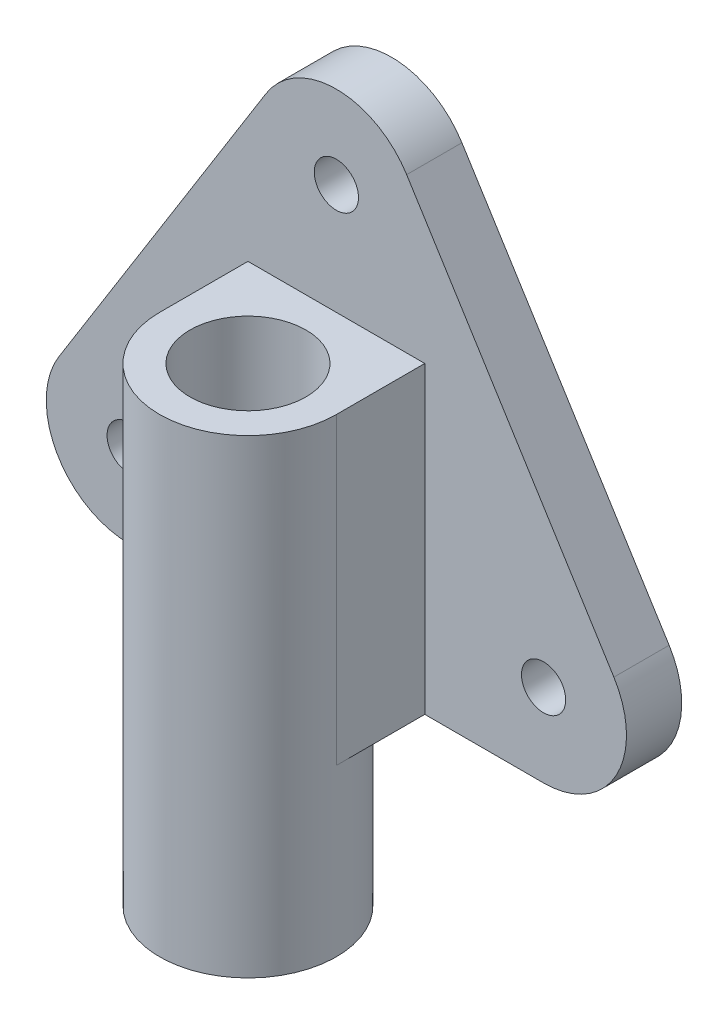
ISO-10303-21;
HEADER;
FILE_DESCRIPTION(('STEP AP214'),'2;1');
FILE_NAME('part.step','',(''),(''),'','','');
FILE_SCHEMA(('AUTOMOTIVE_DESIGN { 1 0 10303 214 1 1 1 1 }'));
ENDSEC;
DATA;
#1=APPLICATION_CONTEXT('core data for automotive mechanical design processes');
#2=APPLICATION_PROTOCOL_DEFINITION('international standard','automotive_design',2000,#1);
#3=PRODUCT_CONTEXT('',#1,'mechanical');
#4=PRODUCT('Part','Part','',(#3));
#5=PRODUCT_RELATED_PRODUCT_CATEGORY('part','',(#4));
#6=PRODUCT_DEFINITION_FORMATION('','',#4);
#7=PRODUCT_DEFINITION_CONTEXT('part definition',#1,'design');
#8=PRODUCT_DEFINITION('design','',#6,#7);
#9=PRODUCT_DEFINITION_SHAPE('','',#8);
#10=(LENGTH_UNIT() NAMED_UNIT(*) SI_UNIT(.MILLI.,.METRE.));
#11=(NAMED_UNIT(*) PLANE_ANGLE_UNIT() SI_UNIT($,.RADIAN.));
#12=(NAMED_UNIT(*) SI_UNIT($,.STERADIAN.) SOLID_ANGLE_UNIT());
#13=UNCERTAINTY_MEASURE_WITH_UNIT(LENGTH_MEASURE(1.E-05),#10,'distance_accuracy_value','');
#14=(GEOMETRIC_REPRESENTATION_CONTEXT(3) GLOBAL_UNCERTAINTY_ASSIGNED_CONTEXT((#13)) GLOBAL_UNIT_ASSIGNED_CONTEXT((#10,
#11,#12)) REPRESENTATION_CONTEXT('',''));
#15=CARTESIAN_POINT('',(0.,0.,0.));
#16=DIRECTION('',(0.,0.,1.));
#17=DIRECTION('',(1.,0.,0.));
#18=AXIS2_PLACEMENT_3D('',#15,#16,#17);
#19=CARTESIAN_POINT('',(0.,-75.,10.));
#20=DIRECTION('',(0.,1.,0.));
#21=DIRECTION('',(0.,0.,1.));
#22=AXIS2_PLACEMENT_3D('',#19,#20,#21);
#23=PLANE('',#22);
#24=CARTESIAN_POINT('',(0.,-75.,26.));
#25=DIRECTION('',(0.,-1.,0.));
#26=DIRECTION('',(0.,0.,-1.));
#27=AXIS2_PLACEMENT_3D('',#24,#25,#26);
#28=CIRCLE('',#27,16.);
#29=CARTESIAN_POINT('',(-16.,-75.,26.));
#30=VERTEX_POINT('',#29);
#31=CARTESIAN_POINT('',(16.,-75.,26.));
#32=VERTEX_POINT('',#31);
#33=EDGE_CURVE('E177',#30,#32,#28,.T.);
#34=ORIENTED_EDGE('',*,*,#33,.F.);
#35=DIRECTION('',(0.,0.,-1.));
#36=VECTOR('',#35,1.);
#37=CARTESIAN_POINT('',(-16.,-75.,0.));
#38=LINE('',#37,#36);
#39=CARTESIAN_POINT('',(-16.,-75.,10.));
#40=VERTEX_POINT('',#39);
#41=EDGE_CURVE('E192',#30,#40,#38,.T.);
#42=ORIENTED_EDGE('',*,*,#41,.T.);
#43=DIRECTION('',(1.,0.,0.));
#44=VECTOR('',#43,1.);
#45=CARTESIAN_POINT('',(0.,-75.,10.));
#46=LINE('',#45,#44);
#47=CARTESIAN_POINT('',(-37.5,-75.,10.));
#48=VERTEX_POINT('',#47);
#49=EDGE_CURVE('E215',#48,#40,#46,.T.);
#50=ORIENTED_EDGE('',*,*,#49,.F.);
#51=DIRECTION('',(0.,0.,-1.));
#52=VECTOR('',#51,1.);
#53=CARTESIAN_POINT('',(-37.5,-75.,10.));
#54=LINE('',#53,#52);
#55=CARTESIAN_POINT('',(-37.5,-75.,0.));
#56=VERTEX_POINT('',#55);
#57=EDGE_CURVE('E140',#48,#56,#54,.T.);
#58=ORIENTED_EDGE('',*,*,#57,.T.);
#59=DIRECTION('',(1.,0.,0.));
#60=VECTOR('',#59,1.);
#61=CARTESIAN_POINT('',(0.,-75.,0.));
#62=LINE('',#61,#60);
#63=CARTESIAN_POINT('',(37.5,-75.,0.));
#64=VERTEX_POINT('',#63);
#65=EDGE_CURVE('E141',#56,#64,#62,.T.);
#66=ORIENTED_EDGE('',*,*,#65,.T.);
#67=DIRECTION('',(0.,0.,-1.));
#68=VECTOR('',#67,1.);
#69=CARTESIAN_POINT('',(37.5,-75.,10.));
#70=LINE('',#69,#68);
#71=CARTESIAN_POINT('',(37.5,-75.,10.));
#72=VERTEX_POINT('',#71);
#73=EDGE_CURVE('E11',#72,#64,#70,.T.);
#74=ORIENTED_EDGE('',*,*,#73,.F.);
#75=CARTESIAN_POINT('',(16.,-75.,10.));
#76=VERTEX_POINT('',#75);
#77=EDGE_CURVE('E102',#76,#72,#46,.T.);
#78=ORIENTED_EDGE('',*,*,#77,.F.);
#79=DIRECTION('',(0.,0.,1.));
#80=VECTOR('',#79,1.);
#81=CARTESIAN_POINT('',(16.,-75.,0.));
#82=LINE('',#81,#80);
#83=EDGE_CURVE('E63',#76,#32,#82,.T.);
#84=ORIENTED_EDGE('',*,*,#83,.T.);
#85=EDGE_LOOP('',(#34,#42,#50,#58,#66,#74,#78,#84));
#86=FACE_BOUND('',#85,.T.);
#87=ADVANCED_FACE('F44',(#86),#23,.F.);
#88=CARTESIAN_POINT('',(37.5,-60.,10.));
#89=DIRECTION('',(0.,0.,-1.));
#90=DIRECTION('',(-1.,0.,0.));
#91=AXIS2_PLACEMENT_3D('',#88,#89,#90);
#92=CYLINDRICAL_SURFACE('',#91,15.);
#93=CARTESIAN_POINT('',(37.5,-60.,0.));
#94=DIRECTION('',(0.,0.,1.));
#95=DIRECTION('',(1.,0.,0.));
#96=AXIS2_PLACEMENT_3D('',#93,#94,#95);
#97=CIRCLE('',#96,15.);
#98=CARTESIAN_POINT('',(50.2199745600763,-52.0500158999523,0.));
#99=VERTEX_POINT('',#98);
#100=EDGE_CURVE('E148',#64,#99,#97,.T.);
#101=ORIENTED_EDGE('',*,*,#100,.T.);
#102=DIRECTION('',(0.,0.,-1.));
#103=VECTOR('',#102,1.);
#104=CARTESIAN_POINT('',(50.2199745600763,-52.0500158999523,10.));
#105=LINE('',#104,#103);
#106=CARTESIAN_POINT('',(50.2199745600763,-52.0500158999523,10.));
#107=VERTEX_POINT('',#106);
#108=EDGE_CURVE('E52',#107,#99,#105,.T.);
#109=ORIENTED_EDGE('',*,*,#108,.F.);
#110=CARTESIAN_POINT('',(37.5,-60.,10.));
#111=DIRECTION('',(0.,0.,1.));
#112=DIRECTION('',(1.,0.,0.));
#113=AXIS2_PLACEMENT_3D('',#110,#111,#112);
#114=CIRCLE('',#113,15.);
#115=EDGE_CURVE('E212',#72,#107,#114,.T.);
#116=ORIENTED_EDGE('',*,*,#115,.F.);
#117=ORIENTED_EDGE('',*,*,#73,.T.);
#118=EDGE_LOOP('',(#101,#109,#116,#117));
#119=FACE_BOUND('',#118,.T.);
#120=ADVANCED_FACE('F236',(#119),#92,.T.);
#121=CARTESIAN_POINT('',(12.7199745600763,7.9499841000477,10.));
#122=DIRECTION('',(0.847998304005088,0.52999894000318,0.));
#123=DIRECTION('',(-0.52999894000318,0.847998304005088,0.));
#124=AXIS2_PLACEMENT_3D('',#121,#122,#123);
#125=PLANE('',#124);
#126=DIRECTION('',(0.52999894000318,-0.847998304005088,0.));
#127=VECTOR('',#126,1.);
#128=CARTESIAN_POINT('',(12.7199745600763,7.9499841000477,0.));
#129=LINE('',#128,#127);
#130=CARTESIAN_POINT('',(12.7199745600763,7.9499841000477,0.));
#131=VERTEX_POINT('',#130);
#132=EDGE_CURVE('E147',#131,#99,#129,.T.);
#133=ORIENTED_EDGE('',*,*,#132,.F.);
#134=DIRECTION('',(0.,0.,-1.));
#135=VECTOR('',#134,1.);
#136=CARTESIAN_POINT('',(12.7199745600763,7.9499841000477,10.));
#137=LINE('',#136,#135);
#138=CARTESIAN_POINT('',(12.7199745600763,7.9499841000477,10.));
#139=VERTEX_POINT('',#138);
#140=EDGE_CURVE('E135',#139,#131,#137,.T.);
#141=ORIENTED_EDGE('',*,*,#140,.F.);
#142=DIRECTION('',(0.52999894000318,-0.847998304005088,0.));
#143=VECTOR('',#142,1.);
#144=CARTESIAN_POINT('',(12.7199745600763,7.9499841000477,10.));
#145=LINE('',#144,#143);
#146=EDGE_CURVE('E122',#139,#107,#145,.T.);
#147=ORIENTED_EDGE('',*,*,#146,.T.);
#148=ORIENTED_EDGE('',*,*,#108,.T.);
#149=EDGE_LOOP('',(#133,#141,#147,#148));
#150=FACE_BOUND('',#149,.T.);
#151=ADVANCED_FACE('F220',(#150),#125,.T.);
#152=CARTESIAN_POINT('',(0.,0.,10.));
#153=DIRECTION('',(0.,0.,-1.));
#154=DIRECTION('',(-1.,0.,0.));
#155=AXIS2_PLACEMENT_3D('',#152,#153,#154);
#156=CYLINDRICAL_SURFACE('',#155,15.);
#157=CARTESIAN_POINT('',(0.,0.,0.));
#158=DIRECTION('',(0.,0.,1.));
#159=DIRECTION('',(1.,0.,0.));
#160=AXIS2_PLACEMENT_3D('',#157,#158,#159);
#161=CIRCLE('',#160,15.);
#162=CARTESIAN_POINT('',(-12.7199745600763,7.9499841000477,0.));
#163=VERTEX_POINT('',#162);
#164=EDGE_CURVE('E128',#131,#163,#161,.T.);
#165=ORIENTED_EDGE('',*,*,#164,.T.);
#166=DIRECTION('',(0.,0.,-1.));
#167=VECTOR('',#166,1.);
#168=CARTESIAN_POINT('',(-12.7199745600763,7.9499841000477,10.));
#169=LINE('',#168,#167);
#170=CARTESIAN_POINT('',(-12.7199745600763,7.9499841000477,10.));
#171=VERTEX_POINT('',#170);
#172=EDGE_CURVE('E130',#171,#163,#169,.T.);
#173=ORIENTED_EDGE('',*,*,#172,.F.);
#174=CARTESIAN_POINT('',(0.,0.,10.));
#175=DIRECTION('',(0.,0.,1.));
#176=DIRECTION('',(1.,0.,0.));
#177=AXIS2_PLACEMENT_3D('',#174,#175,#176);
#178=CIRCLE('',#177,15.);
#179=EDGE_CURVE('E118',#139,#171,#178,.T.);
#180=ORIENTED_EDGE('',*,*,#179,.F.);
#181=ORIENTED_EDGE('',*,*,#140,.T.);
#182=EDGE_LOOP('',(#165,#173,#180,#181));
#183=FACE_BOUND('',#182,.T.);
#184=ADVANCED_FACE('F126',(#183),#156,.T.);
#185=CARTESIAN_POINT('',(-12.7199745600763,7.9499841000477,10.));
#186=DIRECTION('',(-0.847998304005088,0.52999894000318,0.));
#187=DIRECTION('',(-0.52999894000318,-0.847998304005088,0.));
#188=AXIS2_PLACEMENT_3D('',#185,#186,#187);
#189=PLANE('',#188);
#190=DIRECTION('',(0.52999894000318,0.847998304005088,0.));
#191=VECTOR('',#190,1.);
#192=CARTESIAN_POINT('',(-12.7199745600763,7.9499841000477,0.));
#193=LINE('',#192,#191);
#194=CARTESIAN_POINT('',(-50.2199745600763,-52.0500158999523,0.));
#195=VERTEX_POINT('',#194);
#196=EDGE_CURVE('E152',#195,#163,#193,.T.);
#197=ORIENTED_EDGE('',*,*,#196,.F.);
#198=DIRECTION('',(0.,0.,-1.));
#199=VECTOR('',#198,1.);
#200=CARTESIAN_POINT('',(-50.2199745600763,-52.0500158999523,10.));
#201=LINE('',#200,#199);
#202=CARTESIAN_POINT('',(-50.2199745600763,-52.0500158999523,10.));
#203=VERTEX_POINT('',#202);
#204=EDGE_CURVE('E131',#203,#195,#201,.T.);
#205=ORIENTED_EDGE('',*,*,#204,.F.);
#206=DIRECTION('',(0.52999894000318,0.847998304005088,0.));
#207=VECTOR('',#206,1.);
#208=CARTESIAN_POINT('',(-12.7199745600763,7.9499841000477,10.));
#209=LINE('',#208,#207);
#210=EDGE_CURVE('E123',#203,#171,#209,.T.);
#211=ORIENTED_EDGE('',*,*,#210,.T.);
#212=ORIENTED_EDGE('',*,*,#172,.T.);
#213=EDGE_LOOP('',(#197,#205,#211,#212));
#214=FACE_BOUND('',#213,.T.);
#215=ADVANCED_FACE('F139',(#214),#189,.T.);
#216=CARTESIAN_POINT('',(-37.5,-60.,10.));
#217=DIRECTION('',(0.,0.,-1.));
#218=DIRECTION('',(-1.,0.,0.));
#219=AXIS2_PLACEMENT_3D('',#216,#217,#218);
#220=CYLINDRICAL_SURFACE('',#219,15.);
#221=CARTESIAN_POINT('',(-37.5,-60.,0.));
#222=DIRECTION('',(0.,0.,1.));
#223=DIRECTION('',(1.,0.,0.));
#224=AXIS2_PLACEMENT_3D('',#221,#222,#223);
#225=CIRCLE('',#224,15.);
#226=EDGE_CURVE('E100',#195,#56,#225,.T.);
#227=ORIENTED_EDGE('',*,*,#226,.T.);
#228=ORIENTED_EDGE('',*,*,#57,.F.);
#229=CARTESIAN_POINT('',(-37.5,-60.,10.));
#230=DIRECTION('',(0.,0.,1.));
#231=DIRECTION('',(1.,0.,0.));
#232=AXIS2_PLACEMENT_3D('',#229,#230,#231);
#233=CIRCLE('',#232,15.);
#234=EDGE_CURVE('E66',#203,#48,#233,.T.);
#235=ORIENTED_EDGE('',*,*,#234,.F.);
#236=ORIENTED_EDGE('',*,*,#204,.T.);
#237=EDGE_LOOP('',(#227,#228,#235,#236));
#238=FACE_BOUND('',#237,.T.);
#239=ADVANCED_FACE('F228',(#238),#220,.T.);
#240=CARTESIAN_POINT('',(0.,0.,10.));
#241=DIRECTION('',(0.,0.,1.));
#242=DIRECTION('',(1.,0.,0.));
#243=AXIS2_PLACEMENT_3D('',#240,#241,#242);
#244=PLANE('',#243);
#245=CARTESIAN_POINT('',(0.,0.,10.));
#246=DIRECTION('',(0.,0.,1.));
#247=DIRECTION('',(1.,0.,0.));
#248=AXIS2_PLACEMENT_3D('',#245,#246,#247);
#249=CIRCLE('',#248,4.);
#250=CARTESIAN_POINT('',(4.,0.,10.));
#251=VERTEX_POINT('',#250);
#252=EDGE_CURVE('E163',#251,#251,#249,.T.);
#253=ORIENTED_EDGE('',*,*,#252,.F.);
#254=EDGE_LOOP('',(#253));
#255=FACE_BOUND('',#254,.T.);
#256=CARTESIAN_POINT('',(-37.5,-60.,10.));
#257=DIRECTION('',(0.,0.,1.));
#258=DIRECTION('',(1.,0.,0.));
#259=AXIS2_PLACEMENT_3D('',#256,#257,#258);
#260=CIRCLE('',#259,4.);
#261=CARTESIAN_POINT('',(-33.5,-60.,10.));
#262=VERTEX_POINT('',#261);
#263=EDGE_CURVE('E488',#262,#262,#260,.T.);
#264=ORIENTED_EDGE('',*,*,#263,.F.);
#265=EDGE_LOOP('',(#264));
#266=FACE_BOUND('',#265,.T.);
#267=CARTESIAN_POINT('',(37.5,-60.,10.));
#268=DIRECTION('',(0.,0.,1.));
#269=DIRECTION('',(1.,0.,0.));
#270=AXIS2_PLACEMENT_3D('',#267,#268,#269);
#271=CIRCLE('',#270,4.00000000000001);
#272=CARTESIAN_POINT('',(41.5,-60.,10.));
#273=VERTEX_POINT('',#272);
#274=EDGE_CURVE('E491',#273,#273,#271,.T.);
#275=ORIENTED_EDGE('',*,*,#274,.F.);
#276=EDGE_LOOP('',(#275));
#277=FACE_BOUND('',#276,.T.);
#278=DIRECTION('',(0.,-1.,0.));
#279=VECTOR('',#278,1.);
#280=CARTESIAN_POINT('',(-16.,-20.,10.));
#281=LINE('',#280,#279);
#282=CARTESIAN_POINT('',(-16.,-20.,10.));
#283=VERTEX_POINT('',#282);
#284=EDGE_CURVE('E202',#283,#40,#281,.T.);
#285=ORIENTED_EDGE('',*,*,#284,.F.);
#286=DIRECTION('',(-1.,0.,0.));
#287=VECTOR('',#286,1.);
#288=CARTESIAN_POINT('',(0.,-20.,10.));
#289=LINE('',#288,#287);
#290=CARTESIAN_POINT('',(16.,-20.,10.));
#291=VERTEX_POINT('',#290);
#292=EDGE_CURVE('E200',#291,#283,#289,.T.);
#293=ORIENTED_EDGE('',*,*,#292,.F.);
#294=DIRECTION('',(0.,-1.,0.));
#295=VECTOR('',#294,1.);
#296=CARTESIAN_POINT('',(16.,-20.,10.));
#297=LINE('',#296,#295);
#298=EDGE_CURVE('E150',#291,#76,#297,.T.);
#299=ORIENTED_EDGE('',*,*,#298,.T.);
#300=ORIENTED_EDGE('',*,*,#77,.T.);
#301=ORIENTED_EDGE('',*,*,#115,.T.);
#302=ORIENTED_EDGE('',*,*,#146,.F.);
#303=ORIENTED_EDGE('',*,*,#179,.T.);
#304=ORIENTED_EDGE('',*,*,#210,.F.);
#305=ORIENTED_EDGE('',*,*,#234,.T.);
#306=ORIENTED_EDGE('',*,*,#49,.T.);
#307=EDGE_LOOP('',(#285,#293,#299,#300,#301,#302,#303,#304,#305,#306));
#308=FACE_BOUND('',#307,.T.);
#309=ADVANCED_FACE('F120',(#255,#266,#277,#308),#244,.T.);
#310=CARTESIAN_POINT('',(0.,0.,0.));
#311=DIRECTION('',(0.,0.,1.));
#312=DIRECTION('',(1.,0.,0.));
#313=AXIS2_PLACEMENT_3D('',#310,#311,#312);
#314=PLANE('',#313);
#315=CARTESIAN_POINT('',(0.,0.,0.));
#316=DIRECTION('',(0.,0.,1.));
#317=DIRECTION('',(1.,0.,0.));
#318=AXIS2_PLACEMENT_3D('',#315,#316,#317);
#319=CIRCLE('',#318,4.);
#320=CARTESIAN_POINT('',(4.,0.,0.));
#321=VERTEX_POINT('',#320);
#322=EDGE_CURVE('E48',#321,#321,#319,.T.);
#323=ORIENTED_EDGE('',*,*,#322,.T.);
#324=EDGE_LOOP('',(#323));
#325=FACE_BOUND('',#324,.T.);
#326=CARTESIAN_POINT('',(-37.5,-60.,0.));
#327=DIRECTION('',(0.,0.,1.));
#328=DIRECTION('',(1.,0.,0.));
#329=AXIS2_PLACEMENT_3D('',#326,#327,#328);
#330=CIRCLE('',#329,4.);
#331=CARTESIAN_POINT('',(-33.5,-60.,0.));
#332=VERTEX_POINT('',#331);
#333=EDGE_CURVE('E162',#332,#332,#330,.T.);
#334=ORIENTED_EDGE('',*,*,#333,.T.);
#335=EDGE_LOOP('',(#334));
#336=FACE_BOUND('',#335,.T.);
#337=CARTESIAN_POINT('',(37.5,-60.,0.));
#338=DIRECTION('',(0.,0.,1.));
#339=DIRECTION('',(1.,0.,0.));
#340=AXIS2_PLACEMENT_3D('',#337,#338,#339);
#341=CIRCLE('',#340,4.00000000000001);
#342=CARTESIAN_POINT('',(41.5,-60.,0.));
#343=VERTEX_POINT('',#342);
#344=EDGE_CURVE('E161',#343,#343,#341,.T.);
#345=ORIENTED_EDGE('',*,*,#344,.T.);
#346=EDGE_LOOP('',(#345));
#347=FACE_BOUND('',#346,.T.);
#348=ORIENTED_EDGE('',*,*,#65,.F.);
#349=ORIENTED_EDGE('',*,*,#226,.F.);
#350=ORIENTED_EDGE('',*,*,#196,.T.);
#351=ORIENTED_EDGE('',*,*,#164,.F.);
#352=ORIENTED_EDGE('',*,*,#132,.T.);
#353=ORIENTED_EDGE('',*,*,#100,.F.);
#354=EDGE_LOOP('',(#348,#349,#350,#351,#352,#353));
#355=FACE_BOUND('',#354,.T.);
#356=ADVANCED_FACE('F222',(#325,#336,#347,#355),#314,.F.);
#357=CARTESIAN_POINT('',(16.,-20.,0.));
#358=DIRECTION('',(1.,0.,0.));
#359=DIRECTION('',(0.,0.,-1.));
#360=AXIS2_PLACEMENT_3D('',#357,#358,#359);
#361=PLANE('',#360);
#362=ORIENTED_EDGE('',*,*,#83,.F.);
#363=ORIENTED_EDGE('',*,*,#298,.F.);
#364=DIRECTION('',(0.,0.,1.));
#365=VECTOR('',#364,1.);
#366=CARTESIAN_POINT('',(16.,-20.,0.));
#367=LINE('',#366,#365);
#368=CARTESIAN_POINT('',(16.,-20.,26.));
#369=VERTEX_POINT('',#368);
#370=EDGE_CURVE('E205',#291,#369,#367,.T.);
#371=ORIENTED_EDGE('',*,*,#370,.T.);
#372=DIRECTION('',(0.,-1.,0.));
#373=VECTOR('',#372,1.);
#374=CARTESIAN_POINT('',(16.,-20.,26.));
#375=LINE('',#374,#373);
#376=EDGE_CURVE('E193',#369,#32,#375,.T.);
#377=ORIENTED_EDGE('',*,*,#376,.T.);
#378=EDGE_LOOP('',(#362,#363,#371,#377));
#379=FACE_BOUND('',#378,.T.);
#380=ADVANCED_FACE('F279',(#379),#361,.T.);
#381=CARTESIAN_POINT('',(-16.,-20.,0.));
#382=DIRECTION('',(-1.,0.,0.));
#383=DIRECTION('',(0.,0.,1.));
#384=AXIS2_PLACEMENT_3D('',#381,#382,#383);
#385=PLANE('',#384);
#386=ORIENTED_EDGE('',*,*,#41,.F.);
#387=DIRECTION('',(0.,-1.,0.));
#388=VECTOR('',#387,1.);
#389=CARTESIAN_POINT('',(-16.,-20.,26.));
#390=LINE('',#389,#388);
#391=CARTESIAN_POINT('',(-16.,-20.,26.));
#392=VERTEX_POINT('',#391);
#393=EDGE_CURVE('E186',#392,#30,#390,.T.);
#394=ORIENTED_EDGE('',*,*,#393,.F.);
#395=DIRECTION('',(0.,0.,-1.));
#396=VECTOR('',#395,1.);
#397=CARTESIAN_POINT('',(-16.,-20.,0.));
#398=LINE('',#397,#396);
#399=EDGE_CURVE('E198',#392,#283,#398,.T.);
#400=ORIENTED_EDGE('',*,*,#399,.T.);
#401=ORIENTED_EDGE('',*,*,#284,.T.);
#402=EDGE_LOOP('',(#386,#394,#400,#401));
#403=FACE_BOUND('',#402,.T.);
#404=ADVANCED_FACE('F289',(#403),#385,.T.);
#405=CARTESIAN_POINT('',(0.,-20.,0.));
#406=DIRECTION('',(0.,-1.,0.));
#407=DIRECTION('',(0.,0.,-1.));
#408=AXIS2_PLACEMENT_3D('',#405,#406,#407);
#409=PLANE('',#408);
#410=CARTESIAN_POINT('',(0.,-20.,26.));
#411=DIRECTION('',(0.,-1.,0.));
#412=DIRECTION('',(0.,0.,-1.));
#413=AXIS2_PLACEMENT_3D('',#410,#411,#412);
#414=CIRCLE('',#413,10.5);
#415=CARTESIAN_POINT('',(0.,-20.,15.5));
#416=VERTEX_POINT('',#415);
#417=EDGE_CURVE('E172',#416,#416,#414,.T.);
#418=ORIENTED_EDGE('',*,*,#417,.T.);
#419=EDGE_LOOP('',(#418));
#420=FACE_BOUND('',#419,.T.);
#421=ORIENTED_EDGE('',*,*,#399,.F.);
#422=CARTESIAN_POINT('',(0.,-20.,26.));
#423=DIRECTION('',(0.,-1.,0.));
#424=DIRECTION('',(0.,0.,-1.));
#425=AXIS2_PLACEMENT_3D('',#422,#423,#424);
#426=CIRCLE('',#425,16.);
#427=EDGE_CURVE('E183',#369,#392,#426,.T.);
#428=ORIENTED_EDGE('',*,*,#427,.F.);
#429=ORIENTED_EDGE('',*,*,#370,.F.);
#430=ORIENTED_EDGE('',*,*,#292,.T.);
#431=EDGE_LOOP('',(#421,#428,#429,#430));
#432=FACE_BOUND('',#431,.T.);
#433=ADVANCED_FACE('F299',(#420,#432),#409,.F.);
#434=CARTESIAN_POINT('',(0.,-20.,26.));
#435=DIRECTION('',(0.,-1.,0.));
#436=DIRECTION('',(0.,0.,-1.));
#437=AXIS2_PLACEMENT_3D('',#434,#435,#436);
#438=CYLINDRICAL_SURFACE('',#437,16.);
#439=ORIENTED_EDGE('',*,*,#376,.F.);
#440=ORIENTED_EDGE('',*,*,#427,.T.);
#441=ORIENTED_EDGE('',*,*,#393,.T.);
#442=ORIENTED_EDGE('',*,*,#33,.T.);
#443=EDGE_LOOP('',(#439,#440,#441,#442));
#444=FACE_BOUND('',#443,.T.);
#445=CARTESIAN_POINT('',(0.,-105.,26.));
#446=DIRECTION('',(0.,-1.,0.));
#447=DIRECTION('',(0.,0.,-1.));
#448=AXIS2_PLACEMENT_3D('',#445,#446,#447);
#449=CIRCLE('',#448,16.);
#450=CARTESIAN_POINT('',(0.,-105.,10.));
#451=VERTEX_POINT('',#450);
#452=EDGE_CURVE('E185',#451,#451,#449,.T.);
#453=ORIENTED_EDGE('',*,*,#452,.F.);
#454=EDGE_LOOP('',(#453));
#455=FACE_BOUND('',#454,.T.);
#456=ADVANCED_FACE('F307',(#444,#455),#438,.T.);
#457=CARTESIAN_POINT('',(0.,-105.,26.));
#458=DIRECTION('',(0.,-1.,0.));
#459=DIRECTION('',(0.,0.,-1.));
#460=AXIS2_PLACEMENT_3D('',#457,#458,#459);
#461=PLANE('',#460);
#462=CARTESIAN_POINT('',(0.,-105.,26.));
#463=DIRECTION('',(0.,-1.,0.));
#464=DIRECTION('',(0.,0.,-1.));
#465=AXIS2_PLACEMENT_3D('',#462,#463,#464);
#466=CIRCLE('',#465,10.5);
#467=CARTESIAN_POINT('',(0.,-105.,15.5));
#468=VERTEX_POINT('',#467);
#469=EDGE_CURVE('E166',#468,#468,#466,.T.);
#470=ORIENTED_EDGE('',*,*,#469,.F.);
#471=EDGE_LOOP('',(#470));
#472=FACE_BOUND('',#471,.T.);
#473=ORIENTED_EDGE('',*,*,#452,.T.);
#474=EDGE_LOOP('',(#473));
#475=FACE_BOUND('',#474,.T.);
#476=ADVANCED_FACE('F320',(#472,#475),#461,.T.);
#477=CARTESIAN_POINT('',(0.,-20.,26.));
#478=DIRECTION('',(0.,-1.,0.));
#479=DIRECTION('',(0.,0.,-1.));
#480=AXIS2_PLACEMENT_3D('',#477,#478,#479);
#481=CYLINDRICAL_SURFACE('',#480,10.5);
#482=ORIENTED_EDGE('',*,*,#417,.F.);
#483=EDGE_LOOP('',(#482));
#484=FACE_BOUND('',#483,.T.);
#485=ORIENTED_EDGE('',*,*,#469,.T.);
#486=EDGE_LOOP('',(#485));
#487=FACE_BOUND('',#486,.T.);
#488=ADVANCED_FACE('F326',(#484,#487),#481,.F.);
#489=CARTESIAN_POINT('',(37.5,-60.,-75.));
#490=DIRECTION('',(0.,0.,1.));
#491=DIRECTION('',(1.,0.,0.));
#492=AXIS2_PLACEMENT_3D('',#489,#490,#491);
#493=CYLINDRICAL_SURFACE('',#492,4.00000000000001);
#494=ORIENTED_EDGE('',*,*,#274,.T.);
#495=EDGE_LOOP('',(#494));
#496=FACE_BOUND('',#495,.T.);
#497=ORIENTED_EDGE('',*,*,#344,.F.);
#498=EDGE_LOOP('',(#497));
#499=FACE_BOUND('',#498,.T.);
#500=ADVANCED_FACE('F333',(#496,#499),#493,.F.);
#501=CARTESIAN_POINT('',(-37.5,-60.,-75.));
#502=DIRECTION('',(0.,0.,1.));
#503=DIRECTION('',(1.,0.,0.));
#504=AXIS2_PLACEMENT_3D('',#501,#502,#503);
#505=CYLINDRICAL_SURFACE('',#504,4.);
#506=ORIENTED_EDGE('',*,*,#263,.T.);
#507=EDGE_LOOP('',(#506));
#508=FACE_BOUND('',#507,.T.);
#509=ORIENTED_EDGE('',*,*,#333,.F.);
#510=EDGE_LOOP('',(#509));
#511=FACE_BOUND('',#510,.T.);
#512=ADVANCED_FACE('F345',(#508,#511),#505,.F.);
#513=CARTESIAN_POINT('',(0.,0.,-75.));
#514=DIRECTION('',(0.,0.,1.));
#515=DIRECTION('',(1.,0.,0.));
#516=AXIS2_PLACEMENT_3D('',#513,#514,#515);
#517=CYLINDRICAL_SURFACE('',#516,4.);
#518=ORIENTED_EDGE('',*,*,#252,.T.);
#519=EDGE_LOOP('',(#518));
#520=FACE_BOUND('',#519,.T.);
#521=ORIENTED_EDGE('',*,*,#322,.F.);
#522=EDGE_LOOP('',(#521));
#523=FACE_BOUND('',#522,.T.);
#524=ADVANCED_FACE('F355',(#520,#523),#517,.F.);
#525=CLOSED_SHELL('',(#87,#120,#151,#184,#215,#239,#309,#356,#380,#404,#433,#456,#476,#488,#500,
#512,#524));
#526=MANIFOLD_SOLID_BREP('B2',#525);
#527=ADVANCED_BREP_SHAPE_REPRESENTATION('',(#18,#526),#14);
#528=SHAPE_DEFINITION_REPRESENTATION(#9,#527);
ENDSEC;
END-ISO-10303-21;
